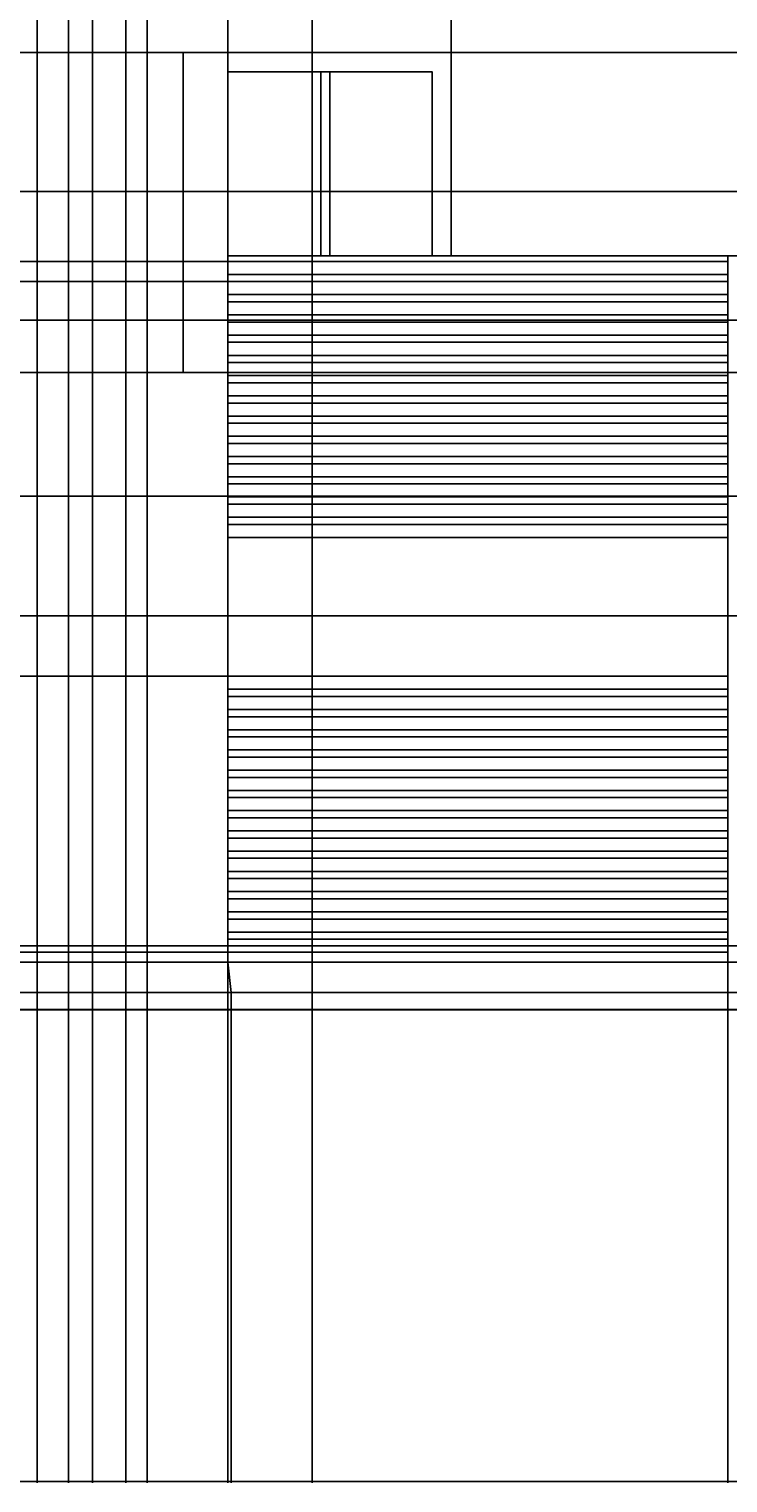
# Model space of a CAD drawing. Units: feet. Extents: x 2193 to 3502, y 890 to 1601.
# Tile 11 of 17: x 3280 to 3369, y 890 to 1076. Entities that reach past the tile are written whole.
import ezdxf

# ---------------------------------------------------------------- set-up
doc = ezdxf.new("R2010")
doc.units = ezdxf.units.FT
doc.layers.add('A-ANNO-DIMS', color=2, linetype='Continuous', lineweight=18)
doc.layers.add('A-ELEV', color=7, linetype='Continuous', lineweight=25)
doc.styles.get("Standard").update_dxf_attribs({"font": 'arial.ttf'})
doc.dimstyles.get("Standard").update_dxf_attribs({"dimtxt": 0.18, "dimasz": 0.18, "dimexe": 0.18, "dimexo": 0.0625, "dimgap": 0.09, "dimtad": 0, "dimtih": 1, "dimtoh": 1, "dimdec": 0, "dimzin": 0, "dimdsep": 46, "dimlunit": 3, "dimtxsty": 'Standard', "dimcen": 0.09, "dimadec": 0, "dimazin": 0, "dimtfac": 1, "dimtdec": 0, "dimtofl": 0, "dimtmove": 0, "dimatfit": 3, "dimfxl": 1, "dimtolj": 1, "dimtzin": 0, "dimarcsym": 0})

# ---------------------------------------------------------------- blocks, each defined once
blk = doc.blocks.new('*D13')
at = {"layer": 'A-ANNO-DIMS', "color": 0, "lineweight": -2, "transparency": 16777216}
for p, q in [((2934.37, 950.89), (2934.37, 1601.47)), ((2934.55, 1601.29), (3186.64, 1601.29)), ((3439.51, 1601.29), (3187.43, 1601.29)), ((3439.69, 1541.11), (3439.69, 1601.47))]:
    blk.add_line(p, q, dxfattribs=at)
at = {"layer": 'A-ANNO-DIMS', "color": 0, "transparency": 16777216}
for points in [[(2934.55, 1601.32), (2934.55, 1601.26), (2934.37, 1601.29)], [(3439.51, 1601.32), (3439.51, 1601.26), (3439.69, 1601.29)]]:
    blk.add_solid(points, dxfattribs=at)
at = {"layer": 'Defpoints', "color": 0, "transparency": 16777216}
for p in [(3439.69, 1601.29), (3439.69, 1541.04), (2934.37, 950.82)]:
    blk.add_point(p, dxfattribs=at)
at = {"layer": 'A-ANNO-DIMS', "color": 0, "transparency": 16777216, "insert": (3187.03, 1601.29), "char_height": 0.18, "attachment_point": 5}
blk.add_mtext('\\A1;505.3', dxfattribs=at)
blk = doc.blocks.new('*D16')
at = {"layer": 'A-ANNO-DIMS', "color": 0, "lineweight": -2, "transparency": 16777216}
for p, q in [((3132, 956.87), (3132, 890.39)), ((3305.41, 950.76), (3305.41, 890.39)), ((3132.18, 890.57), (3218.32, 890.57)), ((3305.23, 890.57), (3219.09, 890.57))]:
    blk.add_line(p, q, dxfattribs=at)
at = {"layer": 'A-ANNO-DIMS', "color": 0, "transparency": 16777216}
for points in [[(3132.18, 890.6), (3132.18, 890.54), (3132, 890.57)], [(3305.23, 890.6), (3305.23, 890.54), (3305.41, 890.57)]]:
    blk.add_solid(points, dxfattribs=at)
at = {"layer": 'Defpoints', "color": 0, "transparency": 16777216}
for p in [(3132, 956.94), (3305.41, 950.82), (3305.41, 890.57)]:
    blk.add_point(p, dxfattribs=at)
at = {"layer": 'A-ANNO-DIMS', "color": 0, "transparency": 16777216, "insert": (3218.71, 890.57), "char_height": 0.18, "attachment_point": 5}
blk.add_mtext('\\A1;173.4', dxfattribs=at)
blk = doc.blocks.new('*D17')
at = {"layer": 'A-ANNO-DIMS', "color": 0, "lineweight": -2, "transparency": 16777216}
for p, q in [((3305.41, 950.76), (3305.41, 890.39)), ((3441.42, 950.76), (3441.42, 890.39)), ((3305.59, 890.57), (3373.14, 890.57)), ((3441.24, 890.57), (3373.7, 890.57))]:
    blk.add_line(p, q, dxfattribs=at)
at = {"layer": 'A-ANNO-DIMS', "color": 0, "transparency": 16777216}
for points in [[(3305.59, 890.6), (3305.59, 890.54), (3305.41, 890.57)], [(3441.24, 890.6), (3441.24, 890.54), (3441.42, 890.57)]]:
    blk.add_solid(points, dxfattribs=at)
at = {"layer": 'Defpoints', "color": 0, "transparency": 16777216}
for p in [(3305.41, 950.82), (3441.42, 950.82), (3441.42, 890.57)]:
    blk.add_point(p, dxfattribs=at)
at = {"layer": 'A-ANNO-DIMS', "color": 0, "transparency": 16777216, "insert": (3373.42, 890.57), "char_height": 0.18, "attachment_point": 5}
blk.add_mtext('\\A1;136', dxfattribs=at)
blk = doc.blocks.new('*D25')
at = {"layer": 'A-ANNO-DIMS', "color": 0, "lineweight": -2, "transparency": 16777216}
for p, q in [((3070.17, 1073.03), (3501.85, 1073.03)), ((3501.67, 1072.85), (3501.67, 1056.13)), ((3501.67, 1039.05), (3501.67, 1055.77)), ((3067.73, 1038.87), (3501.85, 1038.87))]:
    blk.add_line(p, q, dxfattribs=at)
at = {"layer": 'A-ANNO-DIMS', "color": 0, "transparency": 16777216}
for points in [[(3501.64, 1072.85), (3501.7, 1072.85), (3501.67, 1073.03)], [(3501.64, 1039.05), (3501.7, 1039.05), (3501.67, 1038.87)]]:
    blk.add_solid(points, dxfattribs=at)
at = {"layer": 'Defpoints', "color": 0, "transparency": 16777216}
for p in [(3070.11, 1073.03), (3501.67, 1073.03), (3067.66, 1038.87)]:
    blk.add_point(p, dxfattribs=at)
at = {"layer": 'A-ANNO-DIMS', "color": 0, "transparency": 16777216, "insert": (3501.67, 1055.95), "char_height": 0.18, "attachment_point": 5}
blk.add_mtext('\\A1;34.165', dxfattribs=at)
blk = doc.blocks.new('*D31')
at = {"layer": 'A-ANNO-DIMS', "color": 0, "lineweight": -2, "transparency": 16777216}
for p, q in [((2760.54, 1541.04), (3501.85, 1541.04)), ((3501.67, 1540.86), (3501.67, 1246.12)), ((3501.67, 951), (3501.67, 1245.75)), ((2762.27, 950.82), (3501.85, 950.82))]:
    blk.add_line(p, q, dxfattribs=at)
at = {"layer": 'A-ANNO-DIMS', "color": 0, "transparency": 16777216}
for points in [[(3501.64, 1540.86), (3501.7, 1540.86), (3501.67, 1541.04)], [(3501.64, 951), (3501.7, 951), (3501.67, 950.82)]]:
    blk.add_solid(points, dxfattribs=at)
at = {"layer": 'Defpoints', "color": 0, "transparency": 16777216}
for p in [(2760.47, 1541.04), (3501.67, 1541.04), (2762.2, 950.82)]:
    blk.add_point(p, dxfattribs=at)
at = {"layer": 'A-ANNO-DIMS', "color": 0, "transparency": 16777216, "insert": (3501.67, 1245.93), "char_height": 0.18, "attachment_point": 5}
blk.add_mtext('\\A1;590.2', dxfattribs=at)
blk = doc.blocks.new('*D80')
at = {"layer": 'A-ANNO-DIMS', "color": 0, "lineweight": -2, "transparency": 16777216}
for p, q in [((3198.15, 1233.5), (3198.15, 890.39)), ((3315.74, 1233.5), (3315.74, 890.39)), ((3198.33, 890.57), (3256.49, 890.57)), ((3315.56, 890.57), (3257.4, 890.57))]:
    blk.add_line(p, q, dxfattribs=at)
at = {"layer": 'A-ANNO-DIMS', "color": 0, "transparency": 16777216}
for points in [[(3198.33, 890.6), (3198.33, 890.54), (3198.15, 890.57)], [(3315.56, 890.6), (3315.56, 890.54), (3315.74, 890.57)]]:
    blk.add_solid(points, dxfattribs=at)
at = {"layer": 'Defpoints', "color": 0, "transparency": 16777216}
for p in [(3198.15, 1233.56), (3315.74, 1233.56), (3315.74, 890.57)]:
    blk.add_point(p, dxfattribs=at)
at = {"layer": 'A-ANNO-DIMS', "color": 0, "transparency": 16777216, "insert": (3256.94, 890.57), "char_height": 0.18, "attachment_point": 5}
blk.add_mtext('\\A1;117.58', dxfattribs=at)
blk = doc.blocks.new('*D86')
at = {"layer": 'A-ANNO-DIMS', "color": 0, "lineweight": -2, "transparency": 16777216}
for p, q in [((3277.81, 1115.17), (3277.81, 890.39)), ((3280.64, 1112.39), (3280.64, 890.39)), ((3277.99, 890.57), (3278.83, 890.57)), ((3280.46, 890.57), (3279.62, 890.57))]:
    blk.add_line(p, q, dxfattribs=at)
at = {"layer": 'A-ANNO-DIMS', "color": 0, "transparency": 16777216}
for points in [[(3277.99, 890.6), (3277.99, 890.54), (3277.81, 890.57)], [(3280.46, 890.6), (3280.46, 890.54), (3280.64, 890.57)]]:
    blk.add_solid(points, dxfattribs=at)
at = {"layer": 'Defpoints', "color": 0, "transparency": 16777216}
for p in [(3277.81, 1115.23), (3280.64, 1112.45), (3280.64, 890.57)]:
    blk.add_point(p, dxfattribs=at)
at = {"layer": 'A-ANNO-DIMS', "color": 0, "transparency": 16777216, "insert": (3279.22, 890.57), "char_height": 0.18, "attachment_point": 5}
blk.add_mtext('\\A1;2.832', dxfattribs=at)
blk = doc.blocks.new('*D87')
at = {"layer": 'A-ANNO-DIMS', "color": 0, "lineweight": -2, "transparency": 16777216}
for p, q in [((3284.65, 1115.79), (3284.65, 890.39)), ((3280.64, 1112.39), (3280.64, 890.39)), ((3280.82, 890.57), (3282.27, 890.57)), ((3284.47, 890.57), (3283.03, 890.57))]:
    blk.add_line(p, q, dxfattribs=at)
at = {"layer": 'A-ANNO-DIMS', "color": 0, "transparency": 16777216}
for points in [[(3280.82, 890.6), (3280.82, 890.54), (3280.64, 890.57)], [(3284.47, 890.6), (3284.47, 890.54), (3284.65, 890.57)]]:
    blk.add_solid(points, dxfattribs=at)
at = {"layer": 'Defpoints', "color": 0, "transparency": 16777216}
for p in [(3284.65, 1115.85), (3280.64, 1112.45), (3284.65, 890.57)]:
    blk.add_point(p, dxfattribs=at)
at = {"layer": 'A-ANNO-DIMS', "color": 0, "transparency": 16777216, "insert": (3282.65, 890.57), "char_height": 0.18, "attachment_point": 5}
blk.add_mtext('\\A1;4.011', dxfattribs=at)
blk = doc.blocks.new('*D88')
at = {"layer": 'A-ANNO-DIMS', "color": 0, "lineweight": -2, "transparency": 16777216}
for p, q in [((3284.65, 1115.79), (3284.65, 890.39)), ((3287.7, 1113.78), (3287.7, 890.39)), ((3284.83, 890.57), (3285.78, 890.57)), ((3287.52, 890.57), (3286.57, 890.57))]:
    blk.add_line(p, q, dxfattribs=at)
at = {"layer": 'A-ANNO-DIMS', "color": 0, "transparency": 16777216}
for points in [[(3284.83, 890.6), (3284.83, 890.54), (3284.65, 890.57)], [(3287.52, 890.6), (3287.52, 890.54), (3287.7, 890.57)]]:
    blk.add_solid(points, dxfattribs=at)
at = {"layer": 'Defpoints', "color": 0, "transparency": 16777216}
for p in [(3284.65, 1115.85), (3287.7, 1113.84), (3287.7, 890.57)]:
    blk.add_point(p, dxfattribs=at)
at = {"layer": 'A-ANNO-DIMS', "color": 0, "transparency": 16777216, "insert": (3286.18, 890.57), "char_height": 0.18, "attachment_point": 5}
blk.add_mtext('\\A1;3.052', dxfattribs=at)
blk = doc.blocks.new('*D89')
at = {"layer": 'A-ANNO-DIMS', "color": 0, "lineweight": -2, "transparency": 16777216}
for p, q in [((3287.7, 1113.78), (3287.7, 890.39)), ((3291.98, 1108.64), (3291.98, 890.39)), ((3287.88, 890.57), (3289.44, 890.57)), ((3291.8, 890.57), (3290.24, 890.57))]:
    blk.add_line(p, q, dxfattribs=at)
at = {"layer": 'A-ANNO-DIMS', "color": 0, "transparency": 16777216}
for points in [[(3287.88, 890.6), (3287.88, 890.54), (3287.7, 890.57)], [(3291.8, 890.6), (3291.8, 890.54), (3291.98, 890.57)]]:
    blk.add_solid(points, dxfattribs=at)
at = {"layer": 'Defpoints', "color": 0, "transparency": 16777216}
for p in [(3287.7, 1113.84), (3291.98, 1108.7), (3291.98, 890.57)]:
    blk.add_point(p, dxfattribs=at)
at = {"layer": 'A-ANNO-DIMS', "color": 0, "transparency": 16777216, "insert": (3289.84, 890.57), "char_height": 0.18, "attachment_point": 5}
blk.add_mtext('\\A1;4.273', dxfattribs=at)
blk = doc.blocks.new('*D90')
at = {"layer": 'A-ANNO-DIMS', "color": 0, "lineweight": -2, "transparency": 16777216}
for p, q in [((3294.68, 1115), (3294.68, 890.39)), ((3291.98, 1108.64), (3291.98, 890.39)), ((3292.16, 890.57), (3292.93, 890.57)), ((3294.5, 890.57), (3293.72, 890.57))]:
    blk.add_line(p, q, dxfattribs=at)
at = {"layer": 'A-ANNO-DIMS', "color": 0, "transparency": 16777216}
for points in [[(3292.16, 890.6), (3292.16, 890.54), (3291.98, 890.57)], [(3294.5, 890.6), (3294.5, 890.54), (3294.68, 890.57)]]:
    blk.add_solid(points, dxfattribs=at)
at = {"layer": 'Defpoints', "color": 0, "transparency": 16777216}
for p in [(3294.68, 1115.06), (3291.98, 1108.7), (3294.68, 890.57)]:
    blk.add_point(p, dxfattribs=at)
at = {"layer": 'A-ANNO-DIMS', "color": 0, "transparency": 16777216, "insert": (3293.33, 890.57), "char_height": 0.18, "attachment_point": 5}
blk.add_mtext('\\A1;2.703', dxfattribs=at)
blk = doc.blocks.new('*D97')
at = {"layer": 'A-ANNO-DIMS', "color": 0, "lineweight": -2, "transparency": 16777216}
for p, q in [((3111.13, 1032.26), (3111.13, 1601.47)), ((3111.31, 1601.29), (3207.6, 1601.29)), ((3304.79, 1601.29), (3208.51, 1601.29)), ((3304.97, 1032.26), (3304.97, 1601.47))]:
    blk.add_line(p, q, dxfattribs=at)
at = {"layer": 'A-ANNO-DIMS', "color": 0, "transparency": 16777216}
for points in [[(3111.31, 1601.32), (3111.31, 1601.26), (3111.13, 1601.29)], [(3304.79, 1601.32), (3304.79, 1601.26), (3304.97, 1601.29)]]:
    blk.add_solid(points, dxfattribs=at)
at = {"layer": 'Defpoints', "color": 0, "transparency": 16777216}
for p in [(3304.97, 1601.29), (3111.13, 1032.19), (3304.97, 1032.19)]:
    blk.add_point(p, dxfattribs=at)
at = {"layer": 'A-ANNO-DIMS', "color": 0, "transparency": 16777216, "insert": (3208.05, 1601.29), "char_height": 0.18, "attachment_point": 5}
blk.add_mtext('\\A1;193.84', dxfattribs=at)
blk = doc.blocks.new('*D101')
at = {"layer": 'A-ANNO-DIMS', "color": 0, "lineweight": -2, "transparency": 16777216}
for p, q in [((3265.16, 1055.31), (3501.85, 1055.31)), ((3501.67, 1055.13), (3501.67, 1043.93)), ((3501.67, 1032.37), (3501.67, 1043.57)), ((3265.16, 1032.19), (3501.85, 1032.19))]:
    blk.add_line(p, q, dxfattribs=at)
at = {"layer": 'A-ANNO-DIMS', "color": 0, "transparency": 16777216}
for points in [[(3501.64, 1055.13), (3501.7, 1055.13), (3501.67, 1055.31)], [(3501.64, 1032.37), (3501.7, 1032.37), (3501.67, 1032.19)]]:
    blk.add_solid(points, dxfattribs=at)
at = {"layer": 'Defpoints', "color": 0, "transparency": 16777216}
for p in [(3265.1, 1055.31), (3501.67, 1055.31), (3265.1, 1032.19)]:
    blk.add_point(p, dxfattribs=at)
at = {"layer": 'A-ANNO-DIMS', "color": 0, "transparency": 16777216, "insert": (3501.67, 1043.75), "char_height": 0.18, "attachment_point": 5}
blk.add_mtext('\\A1;23.113', dxfattribs=at)
blk = doc.blocks.new('*D103')
at = {"layer": 'A-ANNO-DIMS', "color": 0, "lineweight": -2, "transparency": 16777216}
for p, q in [((3279.67, 1016.4), (3501.85, 1016.4)), ((3501.67, 1016.22), (3501.67, 984.9)), ((3501.67, 953.21), (3501.67, 984.53)), ((3279.67, 953.03), (3501.85, 953.03))]:
    blk.add_line(p, q, dxfattribs=at)
at = {"layer": 'A-ANNO-DIMS', "color": 0, "transparency": 16777216}
for points in [[(3501.64, 1016.22), (3501.7, 1016.22), (3501.67, 1016.4)], [(3501.64, 953.21), (3501.7, 953.21), (3501.67, 953.03)]]:
    blk.add_solid(points, dxfattribs=at)
at = {"layer": 'Defpoints', "color": 0, "transparency": 16777216}
for p in [(3279.61, 1016.4), (3501.67, 1016.4), (3279.61, 953.03)]:
    blk.add_point(p, dxfattribs=at)
at = {"layer": 'A-ANNO-DIMS', "color": 0, "transparency": 16777216, "insert": (3501.67, 984.72), "char_height": 0.18, "attachment_point": 5}
blk.add_mtext('\\A1;63.37', dxfattribs=at)
blk = doc.blocks.new('*D114')
at = {"layer": 'A-ANNO-DIMS', "color": 0, "lineweight": -2, "transparency": 16777216}
for p, q in [((3157.89, 1001.13), (3501.85, 1001.13)), ((3501.67, 1000.95), (3501.67, 980.23)), ((3501.67, 959.14), (3501.67, 979.86)), ((3159.36, 958.96), (3501.85, 958.96))]:
    blk.add_line(p, q, dxfattribs=at)
at = {"layer": 'A-ANNO-DIMS', "color": 0, "transparency": 16777216}
for points in [[(3501.64, 1000.95), (3501.7, 1000.95), (3501.67, 1001.13)], [(3501.64, 959.14), (3501.7, 959.14), (3501.67, 958.96)]]:
    blk.add_solid(points, dxfattribs=at)
at = {"layer": 'Defpoints', "color": 0, "transparency": 16777216}
for p in [(3157.83, 1001.13), (3501.67, 1001.13), (3159.3, 958.96)]:
    blk.add_point(p, dxfattribs=at)
at = {"layer": 'A-ANNO-DIMS', "color": 0, "transparency": 16777216, "insert": (3501.67, 980.04), "char_height": 0.18, "attachment_point": 5}
blk.add_mtext('\\A1;42.18', dxfattribs=at)
blk = doc.blocks.new('*D115')
at = {"layer": 'A-ANNO-DIMS', "color": 0, "lineweight": -2, "transparency": 16777216}
for p, q in [((3192.61, 1016.4), (3501.85, 1016.4)), ((3501.67, 1016.22), (3501.67, 987.86)), ((3501.67, 959.14), (3501.67, 987.5)), ((3194.2, 958.96), (3501.85, 958.96))]:
    blk.add_line(p, q, dxfattribs=at)
at = {"layer": 'A-ANNO-DIMS', "color": 0, "transparency": 16777216}
for points in [[(3501.64, 1016.22), (3501.7, 1016.22), (3501.67, 1016.4)], [(3501.64, 959.14), (3501.7, 959.14), (3501.67, 958.96)]]:
    blk.add_solid(points, dxfattribs=at)
at = {"layer": 'Defpoints', "color": 0, "transparency": 16777216}
for p in [(3192.55, 1016.4), (3501.67, 1016.4), (3194.13, 958.96)]:
    blk.add_point(p, dxfattribs=at)
at = {"layer": 'A-ANNO-DIMS', "color": 0, "transparency": 16777216, "insert": (3501.67, 987.68), "char_height": 0.18, "attachment_point": 5}
blk.add_mtext('\\A1;57.44', dxfattribs=at)
blk = doc.blocks.new('*D121')
at = {"layer": 'A-ANNO-DIMS', "color": 0, "lineweight": -2, "transparency": 16777216}
for p, q in [((3304.97, 956.82), (3304.97, 890.39)), ((3368.82, 956.82), (3368.82, 890.39)), ((3305.15, 890.57), (3336.5, 890.57)), ((3368.64, 890.57), (3337.29, 890.57))]:
    blk.add_line(p, q, dxfattribs=at)
at = {"layer": 'A-ANNO-DIMS', "color": 0, "transparency": 16777216}
for points in [[(3305.15, 890.6), (3305.15, 890.54), (3304.97, 890.57)], [(3368.64, 890.6), (3368.64, 890.54), (3368.82, 890.57)]]:
    blk.add_solid(points, dxfattribs=at)
at = {"layer": 'Defpoints', "color": 0, "transparency": 16777216}
for p in [(3304.97, 956.88), (3368.82, 956.88), (3368.82, 890.57)]:
    blk.add_point(p, dxfattribs=at)
at = {"layer": 'A-ANNO-DIMS', "color": 0, "transparency": 16777216, "insert": (3336.9, 890.57), "char_height": 0.18, "attachment_point": 5}
blk.add_mtext('\\A1;63.84', dxfattribs=at)
blk = doc.blocks.new('*D124')
at = {"layer": 'A-ANNO-DIMS', "color": 0, "lineweight": -2, "transparency": 16777216}
for p, q in [((3304.91, 1046.36), (2193.56, 1046.36)), ((2193.74, 1046.18), (2193.74, 1045.26)), ((3304.91, 1043.78), (2193.56, 1043.78)), ((2193.74, 1043.96), (2193.74, 1044.89))]:
    blk.add_line(p, q, dxfattribs=at)
at = {"layer": 'A-ANNO-DIMS', "color": 0, "transparency": 16777216}
for points in [[(2193.71, 1046.18), (2193.77, 1046.18), (2193.74, 1046.36)], [(2193.71, 1043.96), (2193.77, 1043.96), (2193.74, 1043.78)]]:
    blk.add_solid(points, dxfattribs=at)
at = {"layer": 'Defpoints', "color": 0, "transparency": 16777216}
for p in [(3304.97, 1046.36), (2193.74, 1043.78), (3304.97, 1043.78)]:
    blk.add_point(p, dxfattribs=at)
at = {"layer": 'A-ANNO-DIMS', "color": 0, "transparency": 16777216, "insert": (2193.74, 1045.07), "char_height": 0.18, "attachment_point": 5}
blk.add_mtext('\\A1;2.583', dxfattribs=at)
blk = doc.blocks.new('*D125')
at = {"layer": 'A-ANNO-DIMS', "color": 0, "lineweight": -2, "transparency": 16777216}
for p, q in [((3304.97, 1073.09), (3304.97, 1601.47)), ((3305.15, 1601.29), (3318.84, 1601.29)), ((3333.32, 1601.29), (3319.63, 1601.29)), ((3333.5, 1073.09), (3333.5, 1601.47))]:
    blk.add_line(p, q, dxfattribs=at)
at = {"layer": 'A-ANNO-DIMS', "color": 0, "transparency": 16777216}
for points in [[(3305.15, 1601.32), (3305.15, 1601.26), (3304.97, 1601.29)], [(3333.32, 1601.32), (3333.32, 1601.26), (3333.5, 1601.29)]]:
    blk.add_solid(points, dxfattribs=at)
at = {"layer": 'Defpoints', "color": 0, "transparency": 16777216}
for p in [(3333.5, 1601.29), (3304.97, 1073.03), (3333.5, 1073.03)]:
    blk.add_point(p, dxfattribs=at)
at = {"layer": 'A-ANNO-DIMS', "color": 0, "transparency": 16777216, "insert": (3319.24, 1601.29), "char_height": 0.18, "attachment_point": 5}
blk.add_mtext('\\A1;28.53', dxfattribs=at)
blk = doc.blocks.new('*D130')
at = {"layer": 'A-ANNO-DIMS', "color": 0, "lineweight": -2, "transparency": 16777216}
for p, q in [((3304.91, 993.39), (2193.56, 993.39)), ((2193.74, 993.21), (2193.74, 975.95)), ((2193.74, 958.33), (2193.74, 975.59)), ((3304.91, 958.15), (2193.56, 958.15))]:
    blk.add_line(p, q, dxfattribs=at)
at = {"layer": 'A-ANNO-DIMS', "color": 0, "transparency": 16777216}
for points in [[(2193.71, 993.21), (2193.77, 993.21), (2193.74, 993.39)], [(2193.71, 958.33), (2193.77, 958.33), (2193.74, 958.15)]]:
    blk.add_solid(points, dxfattribs=at)
at = {"layer": 'Defpoints', "color": 0, "transparency": 16777216}
for p in [(2193.74, 993.39), (3304.97, 993.39), (3304.97, 958.15)]:
    blk.add_point(p, dxfattribs=at)
at = {"layer": 'A-ANNO-DIMS', "color": 0, "transparency": 16777216, "insert": (2193.74, 975.77), "char_height": 0.18, "attachment_point": 5}
blk.add_mtext('\\A1;35.24', dxfattribs=at)

msp = doc.modelspace()

# ---------------------------------------------------------------- linework, layer by layer
at = {"layer": 'A-ELEV'}
for p, q in [((2934.3742, 1073.031), (3439.6901, 1073.031)), ((3267.6446, 956.8829), (3304.9731, 956.8829)), ((3305.4139, 953.031), (3304.9731, 956.8829)), ((3305.4139, 950.8228), (3441.4216, 950.8228))]:
    msp.add_line(p, q, dxfattribs=at)
for points in [[(3299.2658, 1032.1935), (3299.2658, 1073.031), (3304.9731, 1073.031), (3304.9731, 956.8829)], [(3304.9731, 1070.5859), (3331.0557, 1070.5859), (3331.0557, 1047.0961)], [(3368.8176, 956.8829), (3368.8176, 1047.0961), (3370.1383, 1047.0961), (3370.1383, 956.8829)], [(3368.8176, 1044.7027), (3304.9731, 1044.7027), (3304.9731, 1046.365), (3368.8176, 1046.365)], [(3368.8176, 1042.1198), (3304.9731, 1042.1198), (3304.9731, 1043.7821), (3368.8176, 1043.7821)], [(3368.8176, 1039.5368), (3304.9731, 1039.5368), (3304.9731, 1041.1991), (3368.8176, 1041.1991)], [(3368.8176, 1036.9539), (3304.9731, 1036.9539), (3304.9731, 1038.6162), (3368.8176, 1038.6162)], [(3368.8176, 1034.371), (3304.9731, 1034.371), (3304.9731, 1036.0333), (3368.8176, 1036.0333)], [(3111.1302, 1016.4), (3111.1302, 1032.1935), (3304.9731, 1032.1935), (3304.9731, 956.8829)], [(3368.8176, 1031.788), (3304.9731, 1031.788), (3304.9731, 1033.4503), (3368.8176, 1033.4503)], [(3368.8176, 1029.2051), (3304.9731, 1029.2051), (3304.9731, 1030.8674), (3368.8176, 1030.8674)], [(3368.8176, 1026.6222), (3304.9731, 1026.6222), (3304.9731, 1028.2844), (3368.8176, 1028.2844)], [(3368.8176, 1024.0392), (3304.9731, 1024.0392), (3304.9731, 1025.7015), (3368.8176, 1025.7015)], [(3368.8176, 1021.4563), (3304.9731, 1021.4563), (3304.9731, 1023.1186), (3368.8176, 1023.1186)], [(3368.8176, 1018.8734), (3304.9731, 1018.8734), (3304.9731, 1020.5356), (3368.8176, 1020.5356)], [(3368.8176, 1016.2904), (3304.9731, 1016.2904), (3304.9731, 1017.9527), (3368.8176, 1017.9527)], [(3368.8176, 1013.7075), (3304.9731, 1013.7075), (3304.9731, 1015.3698), (3368.8176, 1015.3698)], [(3368.8176, 1011.1246), (3304.9731, 1011.1246), (3304.9731, 1012.7868), (3368.8176, 1012.7868)], [(3368.8176, 991.7301), (3304.9731, 991.7301), (3304.9731, 993.3923), (3368.8176, 993.3923)], [(3368.8176, 989.1471), (3304.9731, 989.1471), (3304.9731, 990.8094), (3368.8176, 990.8094)], [(3368.8176, 986.5642), (3304.9731, 986.5642), (3304.9731, 988.2265), (3368.8176, 988.2265)], [(3368.8176, 983.9813), (3304.9731, 983.9813), (3304.9731, 985.6435), (3368.8176, 985.6435)], [(3368.8176, 981.3983), (3304.9731, 981.3983), (3304.9731, 983.0606), (3368.8176, 983.0606)], [(3368.8176, 978.8154), (3304.9731, 978.8154), (3304.9731, 980.4777), (3368.8176, 980.4777)], [(3368.8176, 976.2325), (3304.9731, 976.2325), (3304.9731, 977.8947), (3368.8176, 977.8947)], [(3368.8176, 973.6495), (3304.9731, 973.6495), (3304.9731, 975.3118), (3368.8176, 975.3118)], [(3368.8176, 971.0666), (3304.9731, 971.0666), (3304.9731, 972.7289), (3368.8176, 972.7289)], [(3368.8176, 968.4837), (3304.9731, 968.4837), (3304.9731, 970.1459), (3368.8176, 970.1459)], [(3368.8176, 965.9007), (3304.9731, 965.9007), (3304.9731, 967.563), (3368.8176, 967.563)], [(3368.8176, 963.3178), (3304.9731, 963.3178), (3304.9731, 964.9801), (3368.8176, 964.9801)], [(3368.8176, 960.7348), (3304.9731, 960.7348), (3304.9731, 962.3971), (3368.8176, 962.3971)], [(3368.8176, 958.1519), (3304.9731, 958.1519), (3304.9731, 959.8142), (3368.8176, 959.8142)]]:
    msp.add_lwpolyline(points, dxfattribs=at)
for points in [[(3304.9731, 1073.031), (3333.5009, 1073.031), (3333.5009, 1047.0961), (3304.9731, 1047.0961)], [(3318.0144, 1070.5859), (3316.8485, 1070.5859), (3316.8485, 1047.0961), (3318.0144, 1047.0961)], [(3433.9829, 956.8829), (3304.9731, 956.8829), (3304.9731, 1047.0961), (3433.9829, 1047.0961)], [(2934.3742, 950.8228), (3305.4139, 950.8228), (3305.4139, 953.031), (2934.3742, 953.031)]]:
    msp.add_lwpolyline(points, close=True, dxfattribs=at)

# ---------------------------------------------------------------- dimensions: what is measured, and where the dimension line sits
at = {"layer": 'A-ANNO-DIMS'}
for base, p1, p2, override, picture, middle in [((3439.6901, 1601.2941), (2934.3742, 950.8228), (3439.6901, 1541.0441), {"dimdec": 1, "dimlfac": 1, "dimrnd": 0, "dimzin": 0, "dimdsep": 46, "dimlunit": 2}, '*D13', (3187.0321, 1601.2941)), ((3304.9731, 1601.2941), (3111.1302, 1032.1935), (3304.9731, 1032.1935), {"dimdec": 2, "dimlfac": 1, "dimrnd": 0, "dimzin": 0, "dimdsep": 46, "dimlunit": 2}, '*D97', (3208.0516, 1601.2941)), ((3333.5009, 1601.2941), (3304.9731, 1073.031), (3333.5009, 1073.031), {"dimdec": 2, "dimlfac": 1, "dimrnd": 0, "dimzin": 0, "dimdsep": 46, "dimlunit": 2}, '*D125', (3319.237, 1601.2941)), ((3315.7352, 890.5728), (3198.1547, 1233.561), (3315.7352, 1233.561), {"dimdec": 2, "dimlfac": 1, "dimrnd": 0, "dimzin": 0, "dimdsep": 46, "dimlunit": 2}, '*D80', (3256.9449, 890.5728)), ((3284.651, 890.5728), (3280.6398, 1112.4498), (3284.651, 1115.8479), {"dimdec": 3, "dimlfac": 1, "dimrnd": 0, "dimzin": 0, "dimdsep": 46, "dimlunit": 2}, '*D87', (3282.6454, 890.5728)), ((3287.703, 890.5728), (3284.651, 1115.8479), (3287.703, 1113.8439), {"dimdec": 3, "dimlfac": 1, "dimrnd": 0, "dimzin": 0, "dimdsep": 46, "dimlunit": 2}, '*D88', (3286.177, 890.5728)), ((3280.6398, 890.5728), (3277.8077, 1115.2331), (3280.6398, 1112.4498), {"dimdec": 3, "dimlfac": 1, "dimrnd": 0, "dimzin": 0, "dimdsep": 46, "dimlunit": 2}, '*D86', (3279.2237, 890.5728)), ((3291.9757, 890.5728), (3287.703, 1113.8439), (3291.9757, 1108.7032), {"dimdec": 3, "dimlfac": 1, "dimrnd": 0, "dimzin": 0, "dimdsep": 46, "dimlunit": 2}, '*D89', (3289.8394, 890.5728)), ((3294.679, 890.5728), (3291.9757, 1108.7032), (3294.679, 1115.0637), {"dimdec": 3, "dimlfac": 1, "dimrnd": 0, "dimzin": 0, "dimdsep": 46, "dimlunit": 2}, '*D90', (3293.3274, 890.5728)), ((3305.4139, 890.5728), (3131.9988, 956.9371), (3305.4139, 950.8228), {"dimdec": 1, "dimlfac": 1, "dimrnd": 0, "dimzin": 0, "dimdsep": 46, "dimlunit": 2}, '*D16', (3218.7064, 890.5728)), ((3368.8176, 890.5728), (3304.9731, 956.8829), (3368.8176, 956.8829), {"dimdec": 2, "dimlfac": 1, "dimrnd": 0, "dimzin": 0, "dimdsep": 46, "dimlunit": 2}, '*D121', (3336.8953, 890.5728)), ((3441.4216, 890.5728), (3305.4139, 950.8228), (3441.4216, 950.8228), {"dimdec": 0, "dimlfac": 1, "dimrnd": 0, "dimzin": 0, "dimdsep": 46, "dimlunit": 2}, '*D17', (3373.4177, 890.5728))]:
    dim = msp.add_linear_dim(base=base, p1=p1, p2=p2, dimstyle='Standard', override=override, dxfattribs=at)
    dim.commit()
    dim.dimension.update_dxf_attribs({"geometry": picture, "text_midpoint": middle})
for base, p1, p2, override, picture, middle in [((3501.6716, 1541.0441), (2762.2048, 950.8228), (2760.4733, 1541.0441), {"dimdec": 1, "dimlfac": 1, "dimrnd": 0, "dimzin": 0, "dimdsep": 46, "dimlunit": 2}, '*D31', (3501.6716, 1245.9334)), ((3501.6716, 1073.031), (3067.665, 1038.8658), (3070.1101, 1073.031), {"dimdec": 3, "dimlfac": 1, "dimrnd": 0, "dimzin": 0, "dimdsep": 46, "dimlunit": 2}, '*D25', (3501.6716, 1055.9484)), ((3501.6716, 1055.3069), (3265.1012, 1032.1935), (3265.1012, 1055.3069), {"dimdec": 3, "dimlfac": 1, "dimrnd": 0, "dimzin": 0, "dimdsep": 46, "dimlunit": 2}, '*D101', (3501.6716, 1043.7502)), ((2193.7417, 1043.7821), (3304.9731, 1046.365), (3304.9731, 1043.7821), {"dimdec": 3, "dimlfac": 1, "dimrnd": 0, "dimzin": 0, "dimdsep": 46, "dimlunit": 2}, '*D124', (2193.7417, 1045.0735)), ((3501.6716, 1016.4), (3194.1338, 958.9555), (3192.5464, 1016.4), {"dimdec": 2, "dimlfac": 1, "dimrnd": 0, "dimzin": 0, "dimdsep": 46, "dimlunit": 2}, '*D115', (3501.6716, 987.6777)), ((3501.6716, 1016.4), (3279.6085, 953.031), (3279.6085, 1016.4), {"dimdec": 2, "dimlfac": 1, "dimrnd": 0, "dimzin": 0, "dimdsep": 46, "dimlunit": 2}, '*D103', (3501.6716, 984.7155)), ((3501.6716, 1001.1334), (3159.2977, 958.9555), (3157.8263, 1001.1334), {"dimdec": 2, "dimlfac": 1, "dimrnd": 0, "dimzin": 0, "dimdsep": 46, "dimlunit": 2}, '*D114', (3501.6716, 980.0444)), ((2193.7417, 993.3923), (3304.9731, 958.1519), (3304.9731, 993.3923), {"dimdec": 2, "dimlfac": 1, "dimrnd": 0, "dimzin": 0, "dimdsep": 46, "dimlunit": 2}, '*D130', (2193.7417, 975.7721))]:
    dim = msp.add_linear_dim(base=base, p1=p1, p2=p2, angle=90, dimstyle='Standard', override=override, dxfattribs=at)
    dim.commit()
    dim.dimension.update_dxf_attribs({"geometry": picture, "text_midpoint": middle})

doc.saveas('drawing.dxf')
